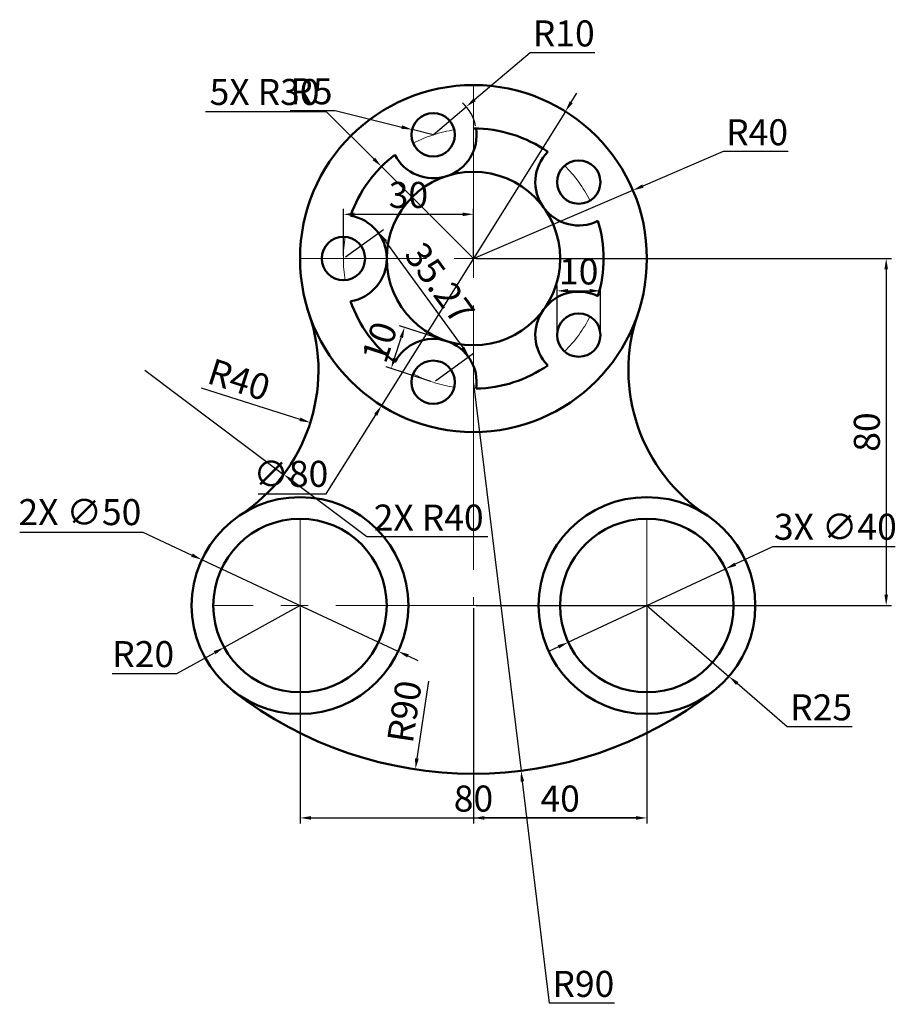
# Model space of a CAD drawing. Units: millimetres. Extents: x -41 to 161, y -105 to 122.
import ezdxf

# ---------------------------------------------------------------- set-up
doc = ezdxf.new("R2010")
doc.units = ezdxf.units.MM
doc.linetypes.add('CENTER', pattern=[50.8, 31.75, -6.35, 6.35, -6.35])
for name, color, linetype, lineweight in [('M-CNTR', 4, 'CENTER', 18), ('M-DIMS', 2, 'Continuous', 25), ('M-OUTL', 7, 'Continuous', 50)]:
    doc.layers.add(name, color=color, linetype=linetype, lineweight=lineweight)
doc.styles.get("Standard").update_dxf_attribs({"font": 'arial.ttf'})
doc.dimstyles.new('ISO-25', dxfattribs={"dimtxt": 6, "dimasz": 2.5, "dimexe": 1.25, "dimexo": 0.625, "dimtad": 1, "dimtoh": 1, "dimdec": 0, "dimtxsty": 'Standard', "dimcen": 2.5, "dimadec": 0, "dimazin": 0, "dimtfac": 1, "dimtdec": 0, "dimtmove": 0, "dimatfit": 3, "dimfxl": 1, "dimarcsym": 0})

# ---------------------------------------------------------------- blocks, each defined once
blk = doc.blocks.new('*U1')
blk.add_circle((0, 0), 5)
blk = doc.blocks.new('*U2')
at = {"layer": 'M-OUTL', "color": 0, "linetype": 'ByBlock', "lineweight": -2, "transparency": 16777216}
for p, rotation in [((54.8, 95.49), 288), ((88.35, 84.59), 216), ((88.35, 49.32), 144), ((54.8, 38.43), 72)]:
    blk.add_blockref('*U1', p, dxfattribs=dict(at, rotation=rotation))
blk.add_blockref('*U1', (34.08, 66.96), dxfattribs=at)
blk = doc.blocks.new('*U3')
blk.add_arc((-5.83, 0), 10, 279.5941, 80.4059)
blk = doc.blocks.new('*U4')
at = {"layer": 'M-OUTL', "color": 0, "linetype": 'ByBlock', "lineweight": -2, "transparency": 16777216}
for p, rotation in [((56.61, 89.94), 288), ((83.63, 81.16), 216), ((83.63, 52.75), 144), ((56.61, 43.97), 72.00000000000001)]:
    blk.add_blockref('*U3', p, dxfattribs=dict(at, rotation=rotation))
blk.add_blockref('*U3', (39.91, 66.96), dxfattribs=at)
blk = doc.blocks.new('*D5')
at = {"layer": 'Defpoints', "color": 0, "transparency": 16777216}
for p in [(100.85, 82.69), (64.08, 66.96)]:
    blk.add_point(p, dxfattribs=at)
at = {"layer": 'M-DIMS', "color": 0, "lineweight": -2, "transparency": 16777216}
for p, q in [((121.7, 91.61), (103.15, 83.67)), ((136.65, 91.61), (121.7, 91.61)), ((64.08, 66.96), (100.85, 82.69))]:
    blk.add_line(p, q, dxfattribs=at)
at = {"layer": 'M-DIMS', "color": 0, "transparency": 16777216}
blk.add_solid([(102.99, 84.05), (103.31, 83.29), (100.85, 82.69)], dxfattribs=at)
at = {"layer": 'M-DIMS', "color": 0, "transparency": 16777216, "insert": (129.49, 95.3), "char_height": 6, "attachment_point": 5}
blk.add_mtext('R40', dxfattribs=at)
blk = doc.blocks.new('*D6')
at = {"layer": 'Defpoints', "color": 0, "transparency": 16777216}
for p in [(49.95, 96.69), (54.8, 95.49)]:
    blk.add_point(p, dxfattribs=at)
at = {"layer": 'M-DIMS', "color": 0, "lineweight": -2, "transparency": 16777216}
for p, q in [((21.84, 101.08), (32.19, 101.08)), ((32.19, 101.08), (47.52, 97.29)), ((54.8, 95.49), (49.95, 96.69))]:
    blk.add_line(p, q, dxfattribs=at)
at = {"layer": 'M-DIMS', "color": 0, "transparency": 16777216}
blk.add_solid([(47.62, 97.69), (47.42, 96.88), (49.95, 96.69)], dxfattribs=at)
at = {"layer": 'M-DIMS', "color": 0, "transparency": 16777216, "insert": (26.7, 104.75), "char_height": 6, "attachment_point": 5}
blk.add_mtext('R5', dxfattribs=at)
blk = doc.blocks.new('*D7')
at = {"layer": 'Defpoints', "color": 0, "transparency": 16777216}
for p in [(62.43, 101.96), (54.8, 95.49)]:
    blk.add_point(p, dxfattribs=at)
at = {"layer": 'M-DIMS', "color": 0, "lineweight": -2, "transparency": 16777216}
for p, q in [((77.12, 114.41), (64.34, 103.57)), ((92.06, 114.41), (77.12, 114.41)), ((54.8, 95.49), (62.43, 101.96))]:
    blk.add_line(p, q, dxfattribs=at)
blk.add_arc((54.8, 95.49), 10, 11.9869, 47.4499, dxfattribs=at)
at = {"layer": 'M-DIMS', "color": 0, "transparency": 16777216}
blk.add_solid([(64.07, 103.89), (64.61, 103.25), (62.43, 101.96)], dxfattribs=at)
at = {"layer": 'M-DIMS', "color": 0, "transparency": 16777216, "insert": (84.9, 118.09), "char_height": 6, "attachment_point": 5}
blk.add_mtext('R10', dxfattribs=at)
blk = doc.blocks.new('*D8')
at = {"layer": 'Defpoints', "color": 0, "transparency": 16777216}
for p in [(-11.68, 41.24), (26.45, 29.14)]:
    blk.add_point(p, dxfattribs=at)
at = {"layer": 'M-DIMS', "color": 0, "lineweight": -2, "transparency": 16777216}
blk.add_line((1.25, 37.14), (24.06, 29.9), dxfattribs=at)
at = {"layer": 'M-DIMS', "color": 0, "transparency": 16777216}
blk.add_solid([(24.19, 30.29), (23.94, 29.5), (26.45, 29.14)], dxfattribs=at)
at = {"layer": 'M-DIMS', "color": 0, "transparency": 16777216, "insert": (9.78, 38.3), "char_height": 6, "attachment_point": 5, "rotation": 342.3937}
blk.add_mtext('R40', dxfattribs=at)
blk = doc.blocks.new('*D9')
at = {"layer": 'Defpoints', "color": 0, "transparency": 16777216}
for p in [(64.08, 38.19), (50.66, -50.8)]:
    blk.add_point(p, dxfattribs=at)
at = {"layer": 'M-DIMS', "color": 0, "lineweight": -2, "transparency": 16777216}
blk.add_line((53.73, -30.47), (51.04, -48.33), dxfattribs=at)
at = {"layer": 'M-DIMS', "color": 0, "transparency": 16777216}
blk.add_solid([(50.62, -48.27), (51.45, -48.39), (50.66, -50.8)], dxfattribs=at)
at = {"layer": 'M-DIMS', "color": 0, "transparency": 16777216, "insert": (48.92, -37.61), "char_height": 6, "attachment_point": 5, "rotation": 81.43}
blk.add_mtext('R90', dxfattribs=at)
blk = doc.blocks.new('*D10')
at = {"layer": 'Defpoints', "color": 0, "transparency": 16777216}
for p in [(104.08, -13.04), (123, -29.38)]:
    blk.add_point(p, dxfattribs=at)
at = {"layer": 'M-DIMS', "color": 0, "lineweight": -2, "transparency": 16777216}
for p, q in [((104.08, -13.04), (123, -29.38)), ((136.45, -40.98), (124.89, -31.01)), ((151.45, -40.98), (136.45, -40.98))]:
    blk.add_line(p, q, dxfattribs=at)
at = {"layer": 'M-DIMS', "color": 0, "transparency": 16777216}
blk.add_solid([(125.17, -30.69), (124.62, -31.33), (123, -29.38)], dxfattribs=at)
at = {"layer": 'M-DIMS', "color": 0, "transparency": 16777216, "insert": (144.26, -37.29), "char_height": 6, "attachment_point": 5}
blk.add_mtext('R25', dxfattribs=at)
blk = doc.blocks.new('*D11')
at = {"layer": 'Defpoints', "color": 0, "transparency": 16777216}
for p in [(24.08, -13.04), (6.56, -22.7)]:
    blk.add_point(p, dxfattribs=at)
at = {"layer": 'M-DIMS', "color": 0, "lineweight": -2, "transparency": 16777216}
for p, q in [((24.08, -13.04), (6.56, -22.7)), ((-4.32, -28.7), (4.37, -23.91)), ((-19.26, -28.7), (-4.32, -28.7))]:
    blk.add_line(p, q, dxfattribs=at)
at = {"layer": 'M-DIMS', "color": 0, "transparency": 16777216}
blk.add_solid([(4.17, -23.54), (4.57, -24.27), (6.56, -22.7)], dxfattribs=at)
at = {"layer": 'M-DIMS', "color": 0, "transparency": 16777216, "insert": (-12.1, -25.02), "char_height": 6, "attachment_point": 5}
blk.add_mtext('R20', dxfattribs=at)
blk = doc.blocks.new('*D12')
at = {"layer": 'Defpoints', "color": 0, "transparency": 16777216}
for p in [(64.08, 66.96), (64.08, -13.04), (159.27, -13.04)]:
    blk.add_point(p, dxfattribs=at)
at = {"layer": 'M-DIMS', "color": 0, "lineweight": -2, "transparency": 16777216}
for p, q in [((64.7, 66.96), (160.52, 66.96)), ((159.27, 64.46), (159.27, -10.54)), ((64.7, -13.04), (160.52, -13.04))]:
    blk.add_line(p, q, dxfattribs=at)
at = {"layer": 'M-DIMS', "color": 0, "transparency": 16777216}
for points in [[(158.85, 64.46), (159.68, 64.46), (159.27, 66.96)], [(158.85, -10.54), (159.68, -10.54), (159.27, -13.04)]]:
    blk.add_solid(points, dxfattribs=at)
at = {"layer": 'M-DIMS', "color": 0, "transparency": 16777216, "insert": (155.58, 26.96), "char_height": 6, "attachment_point": 5, "rotation": 90}
blk.add_mtext('80', dxfattribs=at)
blk = doc.blocks.new('LINK-BOSS-OD50-ID40')
for radius in [25, 20]:
    blk.add_circle((0, 0), radius)
blk = doc.blocks.new('*D14')
at = {"layer": 'Defpoints', "color": 0, "transparency": 16777216}
for p in [(24.08, -13.04), (104.08, -13.04), (104.08, -62.01)]:
    blk.add_point(p, dxfattribs=at)
at = {"layer": 'M-DIMS', "color": 0, "lineweight": -2, "transparency": 16777216}
for p, q in [((24.08, -13.67), (24.08, -63.26)), ((104.08, -13.67), (104.08, -63.26)), ((26.58, -62.01), (101.58, -62.01))]:
    blk.add_line(p, q, dxfattribs=at)
at = {"layer": 'M-DIMS', "color": 0, "transparency": 16777216}
for points in [[(26.58, -61.59), (26.58, -62.42), (24.08, -62.01)], [(101.58, -61.59), (101.58, -62.42), (104.08, -62.01)]]:
    blk.add_solid(points, dxfattribs=at)
at = {"layer": 'M-DIMS', "color": 0, "transparency": 16777216, "insert": (64.08, -58.32), "char_height": 6, "attachment_point": 5}
blk.add_mtext('80', dxfattribs=at)
blk = doc.blocks.new('*D15')
at = {"layer": 'Defpoints', "color": 0, "transparency": 16777216}
for p in [(64.08, -13.04), (104.08, -13.04), (64.08, -62.01)]:
    blk.add_point(p, dxfattribs=at)
at = {"layer": 'M-DIMS', "color": 0, "lineweight": -2, "transparency": 16777216}
for p, q in [((64.08, -13.67), (64.08, -63.26)), ((104.08, -13.67), (104.08, -63.26)), ((101.58, -62.01), (66.58, -62.01))]:
    blk.add_line(p, q, dxfattribs=at)
at = {"layer": 'M-DIMS', "color": 0, "transparency": 16777216}
for points in [[(66.58, -61.59), (66.58, -62.42), (64.08, -62.01)], [(101.58, -61.59), (101.58, -62.42), (104.08, -62.01)]]:
    blk.add_solid(points, dxfattribs=at)
at = {"layer": 'M-DIMS', "color": 0, "transparency": 16777216, "insert": (84.08, -58.32), "char_height": 6, "attachment_point": 5}
blk.add_mtext('40', dxfattribs=at)
blk = doc.blocks.new('*D16')
at = {"layer": 'Defpoints', "color": 0, "transparency": 16777216}
for p in [(93.35, 59.52), (83.35, 49.32), (93.35, 49.32)]:
    blk.add_point(p, dxfattribs=at)
at = {"layer": 'M-DIMS', "color": 0, "lineweight": -2, "transparency": 16777216}
for p, q in [((83.35, 49.95), (83.35, 60.77)), ((85.85, 59.52), (90.85, 59.52)), ((93.35, 49.95), (93.35, 60.77))]:
    blk.add_line(p, q, dxfattribs=at)
at = {"layer": 'M-DIMS', "color": 0, "transparency": 16777216}
for points in [[(85.85, 59.94), (85.85, 59.11), (83.35, 59.52)], [(90.85, 59.94), (90.85, 59.11), (93.35, 59.52)]]:
    blk.add_solid(points, dxfattribs=at)
at = {"layer": 'M-DIMS', "color": 0, "transparency": 16777216, "insert": (88.35, 63.21), "char_height": 6, "attachment_point": 5}
blk.add_mtext('10', dxfattribs=at)
blk = doc.blocks.new('*D17')
at = {"layer": 'Defpoints', "color": 0, "transparency": 16777216}
for p in [(48.19, 51.09), (57.89, 47.94), (54.8, 38.43)]:
    blk.add_point(p, dxfattribs=at)
at = {"layer": 'M-DIMS', "color": 0, "lineweight": -2, "transparency": 16777216}
for p, q in [((57.3, 48.13), (47.01, 51.47)), ((45.88, 43.96), (47.42, 48.71)), ((54.21, 38.62), (43.92, 41.96))]:
    blk.add_line(p, q, dxfattribs=at)
at = {"layer": 'M-DIMS', "color": 0, "transparency": 16777216}
for points in [[(47.03, 48.84), (47.82, 48.58), (48.19, 51.09)], [(45.48, 44.08), (46.27, 43.83), (45.1, 41.58)]]:
    blk.add_solid(points, dxfattribs=at)
at = {"layer": 'M-DIMS', "color": 0, "transparency": 16777216, "insert": (43.14, 47.47), "char_height": 6, "attachment_point": 5, "rotation": 72}
blk.add_mtext('10', dxfattribs=at)
blk = doc.blocks.new('*D18')
at = {"layer": 'Defpoints', "color": 0, "transparency": 16777216}
for p in [(64.08, 77.16), (34.08, 66.96), (64.08, 66.96)]:
    blk.add_point(p, dxfattribs=at)
at = {"layer": 'M-DIMS', "color": 0, "lineweight": -2, "transparency": 16777216}
for p, q in [((34.08, 67.58), (34.08, 78.41)), ((64.08, 67.58), (64.08, 78.41)), ((36.58, 77.16), (61.58, 77.16))]:
    blk.add_line(p, q, dxfattribs=at)
at = {"layer": 'M-DIMS', "color": 0, "transparency": 16777216}
for points in [[(36.58, 77.57), (36.58, 76.74), (34.08, 77.16)], [(61.58, 77.57), (61.58, 76.74), (64.08, 77.16)]]:
    blk.add_solid(points, dxfattribs=at)
at = {"layer": 'M-DIMS', "color": 0, "transparency": 16777216, "insert": (49.08, 80.85), "char_height": 6, "attachment_point": 5}
blk.add_mtext('30', dxfattribs=at)
blk = doc.blocks.new('*D19')
at = {"layer": 'Defpoints', "color": 0, "transparency": 16777216}
for p in [(34.08, 66.96), (63.06, 44.42), (54.8, 38.43)]:
    blk.add_point(p, dxfattribs=at)
at = {"layer": 'M-DIMS', "color": 0, "lineweight": -2, "transparency": 16777216}
for p, q in [((34.58, 67.32), (43.34, 73.69)), ((43.8, 70.93), (61.59, 46.44)), ((55.31, 38.79), (64.07, 45.16))]:
    blk.add_line(p, q, dxfattribs=at)
at = {"layer": 'M-DIMS', "color": 0, "transparency": 16777216}
for points in [[(44.13, 71.17), (43.46, 70.69), (42.33, 72.95)], [(61.92, 46.69), (61.25, 46.2), (63.06, 44.42)]]:
    blk.add_solid(points, dxfattribs=at)
at = {"layer": 'M-DIMS', "color": 0, "transparency": 16777216, "insert": (55.68, 60.86), "char_height": 6, "attachment_point": 5, "rotation": 306}
blk.add_mtext('35.27', dxfattribs=at)
blk = doc.blocks.new('*D20')
at = {"layer": 'Defpoints', "color": 0, "transparency": 16777216}
for p in [(64.08, 38.19), (75.05, -51.14)]:
    blk.add_point(p, dxfattribs=at)
at = {"layer": 'M-DIMS', "color": 0, "lineweight": -2, "transparency": 16777216}
for p, q in [((64.08, 38.19), (75.05, -51.14)), ((81.63, -104.73), (75.35, -53.62)), ((96.58, -104.73), (81.63, -104.73))]:
    blk.add_line(p, q, dxfattribs=at)
at = {"layer": 'M-DIMS', "color": 0, "transparency": 16777216}
blk.add_solid([(75.77, -53.57), (74.94, -53.67), (75.05, -51.14)], dxfattribs=at)
at = {"layer": 'M-DIMS', "color": 0, "transparency": 16777216, "insert": (89.42, -101.05), "char_height": 6, "attachment_point": 5}
blk.add_mtext('R90', dxfattribs=at)
blk = doc.blocks.new('*D21')
at = {"layer": 'Defpoints', "color": 0, "transparency": 16777216}
for p in [(-11.68, 41.24), (20.29, 17.2)]:
    blk.add_point(p, dxfattribs=at)
at = {"layer": 'M-DIMS', "color": 0, "lineweight": -2, "transparency": 16777216}
for p, q in [((-11.68, 41.24), (20.29, 17.2)), ((39.47, 2.77), (22.29, 15.69)), ((67.4, 2.77), (39.47, 2.77))]:
    blk.add_line(p, q, dxfattribs=at)
at = {"layer": 'M-DIMS', "color": 0, "transparency": 16777216}
blk.add_solid([(22.54, 16.03), (22.04, 15.36), (20.29, 17.2)], dxfattribs=at)
at = {"layer": 'M-DIMS', "color": 0, "transparency": 16777216, "insert": (53.75, 6.46), "char_height": 6, "attachment_point": 5}
blk.add_mtext('2X R40', dxfattribs=at)
blk = doc.blocks.new('*D22')
at = {"layer": 'Defpoints', "color": 0, "transparency": 16777216}
for p in [(1.42, -2.48), (46.73, -23.61)]:
    blk.add_point(p, dxfattribs=at)
at = {"layer": 'M-DIMS', "color": 0, "lineweight": -2, "transparency": 16777216}
for p, q in [((-40.58, 3.86), (-12.18, 3.86)), ((-12.18, 3.86), (-0.85, -1.42)), ((46.73, -23.61), (1.42, -2.48)), ((49, -24.67), (51.26, -25.72))]:
    blk.add_line(p, q, dxfattribs=at)
at = {"layer": 'M-DIMS', "color": 0, "transparency": 16777216}
for points in [[(-0.67, -1.04), (-1.02, -1.8), (1.42, -2.48)], [(49.17, -24.29), (48.82, -25.04), (46.73, -23.61)]]:
    blk.add_solid(points, dxfattribs=at)
at = {"layer": 'M-DIMS', "color": 0, "transparency": 16777216, "insert": (-26.69, 7.72), "char_height": 6, "attachment_point": 5}
blk.add_mtext('2X ∅50', dxfattribs=at)
blk = doc.blocks.new('*D23')
at = {"layer": 'Defpoints', "color": 0, "transparency": 16777216}
for p in [(122.2, -4.59), (85.95, -21.5)]:
    blk.add_point(p, dxfattribs=at)
at = {"layer": 'M-DIMS', "color": 0, "lineweight": -2, "transparency": 16777216}
for p, q in [((133.08, 0.48), (124.47, -3.53)), ((161.37, 0.48), (133.08, 0.48)), ((85.95, -21.5), (122.2, -4.59)), ((83.68, -22.55), (81.42, -23.61))]:
    blk.add_line(p, q, dxfattribs=at)
at = {"layer": 'M-DIMS', "color": 0, "transparency": 16777216}
for points in [[(124.29, -3.16), (124.64, -3.91), (122.2, -4.59)], [(83.51, -22.18), (83.86, -22.93), (85.95, -21.5)]]:
    blk.add_solid(points, dxfattribs=at)
at = {"layer": 'M-DIMS', "color": 0, "transparency": 16777216, "insert": (147.54, 4.34), "char_height": 6, "attachment_point": 5}
blk.add_mtext('3X ∅40', dxfattribs=at)
blk = doc.blocks.new('*D24')
at = {"layer": 'Defpoints', "color": 0, "transparency": 16777216}
for p in [(85.29, 100.87), (42.86, 33.05)]:
    blk.add_point(p, dxfattribs=at)
at = {"layer": 'M-DIMS', "color": 0, "lineweight": -2, "transparency": 16777216}
for p, q in [((86.61, 102.99), (87.94, 105.11)), ((85.29, 100.87), (42.86, 33.05)), ((30.13, 12.7), (41.54, 30.93)), ((14.41, 12.7), (30.13, 12.7))]:
    blk.add_line(p, q, dxfattribs=at)
at = {"layer": 'M-DIMS', "color": 0, "transparency": 16777216}
for points in [[(86.26, 103.21), (86.97, 102.77), (85.29, 100.87)], [(41.18, 31.15), (41.89, 30.71), (42.86, 33.05)]]:
    blk.add_solid(points, dxfattribs=at)
at = {"layer": 'M-DIMS', "color": 0, "transparency": 16777216, "insert": (21.96, 16.55), "char_height": 6, "attachment_point": 5}
blk.add_mtext('∅80', dxfattribs=at)
blk = doc.blocks.new('*D25')
at = {"layer": 'Defpoints', "color": 0, "transparency": 16777216}
for p in [(42.86, 88.17), (64.08, 66.96)]:
    blk.add_point(p, dxfattribs=at)
at = {"layer": 'M-DIMS', "color": 0, "lineweight": -2, "transparency": 16777216}
for p, q in [((2.3, 100.9), (30.13, 100.9)), ((30.13, 100.9), (41.09, 89.94)), ((64.08, 66.96), (42.86, 88.17))]:
    blk.add_line(p, q, dxfattribs=at)
at = {"layer": 'M-DIMS', "color": 0, "transparency": 16777216}
blk.add_solid([(41.39, 90.23), (40.8, 89.64), (42.86, 88.17)], dxfattribs=at)
at = {"layer": 'M-DIMS', "color": 0, "transparency": 16777216, "insert": (15.9, 104.59), "char_height": 6, "attachment_point": 5}
blk.add_mtext('5X R30', dxfattribs=at)

msp = doc.modelspace()

# ---------------------------------------------------------------- linework, layer by layer
at = {"layer": 'M-CNTR'}
for p, q in [((104.075, 66.957), (24.075, 66.957)), ((24.075, 6.957), (24.075, -33.043)), ((104.075, 6.957), (104.075, -33.043)), ((64.075, -13.043), (4.075, -13.043)), ((64.075, -13.043), (124.075, -13.043))]:
    msp.add_line(p, q, dxfattribs=at)
msp.add_lwpolyline([(64.075, 106.957), (64.075, 26.957), (64.075, -13.043)], dxfattribs=at)
for start, end in [(98.43962, 117.56038), (26.43962, 45.56038), (170.43962, 189.56038), (314.43962, 333.56038), (242.43962, 261.56038)]:
    msp.add_arc((64.075, 66.957), 30, start, end, dxfattribs=at)
at = {"layer": 'M-OUTL'}
for radius in [40, 20]:
    msp.add_circle((64.075, 66.957), radius, dxfattribs=at)
for centre, radius, start, end in [((64.075, 66.957), 30, 55.18814, 90), ((64.075, 66.957), 30, 127.18814, 160.81186), ((64.075, 66.957), 30, 343.18814, 16.81186), ((64.075, 66.957), 30, 199.18814, 232.81186), ((-12.188, 42.837), 40, 16.50882, 18.59231), ((-11.679, 41.24), 40, 303.37107, 18.75126), ((139.829, 41.24), 40, 161.24874, 236.62893), ((64.075, 66.957), 30, 271.18814, 304.81186), ((64.075, 38.192), 90, 232.02013, 307.97987)]:
    msp.add_arc(centre, radius, start, end, dxfattribs=at)

# ---------------------------------------------------------------- block references
for name, p in [('*U2', (0, 0)), ('*U4', (0, 0)), ('LINK-BOSS-OD50-ID40', (24.075, -13.043)), ('LINK-BOSS-OD50-ID40', (104.075, -13.043))]:
    msp.add_blockref(name, p, dxfattribs=at)

# ---------------------------------------------------------------- dimensions: what is measured, and where the dimension line sits
at = {"layer": 'M-DIMS'}
for center, mpoint, override, picture, middle in [((54.805, 95.489), (62.433, 101.955), {"dimclrd": 0, "dimclre": 0, "dimclrt": 0}, '*D7', (84.904, 114.406)), ((54.805, 95.489), (49.951, 96.688), {"dimclrd": 0, "dimclre": 0, "dimclrt": 0}, '*D6', (32.187, 101.078)), ((64.075, 66.957), (100.852, 82.688), {"dimclrd": 0, "dimclre": 0, "dimclrt": 0}, '*D5', (129.487, 91.607)), ((-11.679, 41.24), (26.448, 29.141), {"dimclrd": 0, "dimclre": 0, "dimclrt": 0}, '*D8', (8.667, 34.784)), ((64.075, 38.192), (50.664, -50.803), {"dimclrd": 0, "dimclre": 0, "dimclrt": 0}, '*D9', (52.568, -38.163)), ((64.075, 38.192), (75.05, -51.136), {"dimdec": 0, "dimlfac": 1, "dimrnd": 0, "dimzin": 0, "dimdsep": 46, "dimlunit": 2}, '*D20', (89.417, -104.733)), ((24.075, -13.043), (6.562, -22.701), {"dimclrd": 0, "dimclre": 0, "dimclrt": 0}, '*D11', (-12.105, -28.704)), ((104.075, -13.043), (123.002, -29.376), {"dimclrd": 0, "dimclre": 0, "dimclrt": 0}, '*D10', (144.263, -40.98))]:
    dim = msp.add_radius_dim(center=center, mpoint=mpoint, dimstyle='ISO-25', override=override, dxfattribs=at)
    dim.commit()
    dim.dimension.update_dxf_attribs({"geometry": picture, "text_midpoint": middle, "dimtype": 164})
for center, mpoint, text, picture, middle in [((64.075, 66.957), (42.862, 88.17), '5X <>', '*D25', (15.904, 100.898)), ((-11.679, 41.24), (20.288, 17.197), '2X <>', '*D21', (53.749, 2.77))]:
    dim = msp.add_radius_dim(center=center, mpoint=mpoint, text=text, dimstyle='ISO-25', override={"dimdec": 0, "dimlfac": 1, "dimrnd": 0, "dimzin": 0, "dimdsep": 46, "dimlunit": 2}, dxfattribs=at)
    dim.commit()
    dim.dimension.update_dxf_attribs({"geometry": picture, "text_midpoint": middle, "dimtype": 164})
dim = msp.add_diameter_dim_2p(p1=(85.288, 100.869), p2=(42.862, 33.046), dimstyle='ISO-25', override={"dimdec": 0, "dimlfac": 1, "dimrnd": 0, "dimzin": 0, "dimdsep": 46, "dimlunit": 2}, dxfattribs=at)
dim.commit()
dim.dimension.update_dxf_attribs({"geometry": '*D24', "text_midpoint": (21.958, 12.699), "dimtype": 163})
for base, p1, p2, picture, middle in [((64.075, 77.157), (34.075, 66.957), (64.075, 66.957), '*D18', (49.075, 80.848)), ((93.346, 59.524), (83.346, 49.324), (93.346, 49.324), '*D16', (88.346, 63.212)), ((104.075, -62.008), (24.075, -13.043), (104.075, -13.043), '*D14', (64.075, -58.32)), ((64.075, -62.008), (104.075, -13.043), (64.075, -13.043), '*D15', (84.075, -58.32))]:
    dim = msp.add_linear_dim(base=base, p1=p1, p2=p2, dimstyle='ISO-25', override={"dimdec": 0, "dimlfac": 1, "dimrnd": 0, "dimzin": 0, "dimdsep": 46, "dimlunit": 2}, dxfattribs=at)
    dim.commit()
    dim.dimension.update_dxf_attribs({"geometry": picture, "text_midpoint": middle})
for base, p1, p2, angle, override, picture, middle in [((63.057, 44.421), (34.075, 66.957), (54.805, 38.425), 306, {"dimdec": 2, "dimlfac": 1, "dimrnd": 0, "dimzin": 0, "dimdsep": 46, "dimlunit": 2}, '*D19', (55.678, 60.856)), ((159.265, -13.043), (64.075, 66.957), (64.075, -13.043), 90, {"dimclrd": 0, "dimclre": 0, "dimclrt": 0}, '*D12', (155.577, 26.957)), ((48.194, 51.088), (54.805, 38.425), (57.895, 47.936), 72, {"dimdec": 0, "dimlfac": 1, "dimrnd": 0, "dimzin": 0, "dimdsep": 46, "dimlunit": 2}, '*D17', (43.141, 47.473))]:
    dim = msp.add_linear_dim(base=base, p1=p1, p2=p2, angle=angle, dimstyle='ISO-25', override=override, dxfattribs=at)
    dim.commit()
    dim.dimension.update_dxf_attribs({"geometry": picture, "text_midpoint": middle})
for p1, p2, text, picture, middle in [((46.733, -23.609), (1.418, -2.477), '2X <>', '*D22', (-26.691, 3.863)), ((85.949, -21.496), (122.201, -4.59), '3X <>', '*D23', (147.537, 0.482))]:
    dim = msp.add_diameter_dim_2p(p1=p1, p2=p2, text=text, dimstyle='ISO-25', override={"dimdec": 0, "dimlfac": 1, "dimrnd": 0, "dimzin": 0, "dimdsep": 46, "dimlunit": 2}, dxfattribs=at)
    dim.commit()
    dim.dimension.update_dxf_attribs({"geometry": picture, "text_midpoint": middle, "dimtype": 163})

doc.saveas('drawing.dxf')
